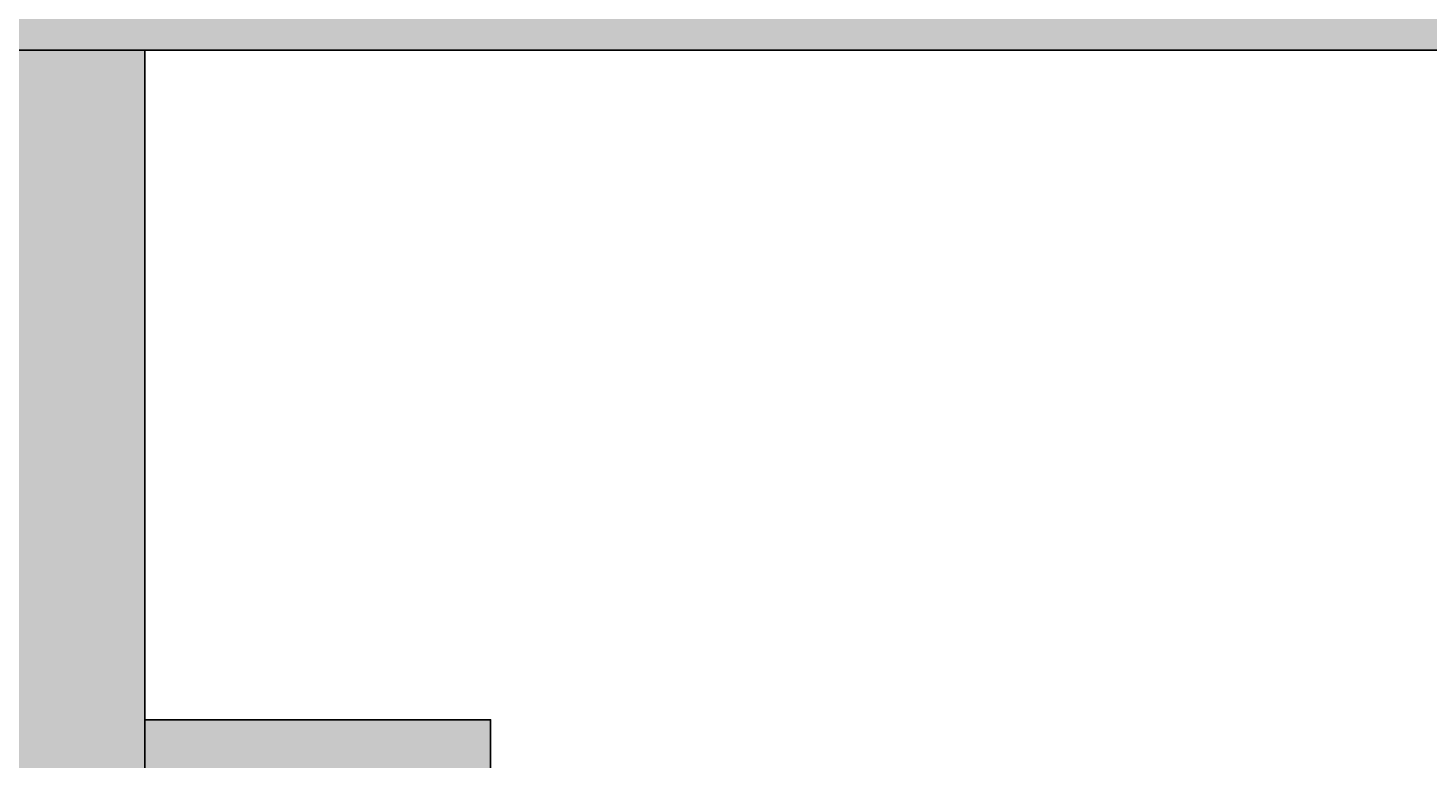
# Model space of a CAD drawing. Units: millimetres. Extents: x -11 to 280, y -4 to 208.
# Tile 34 of 55: x 189 to 222, y 88 to 106. Entities that reach past the tile are written whole.
import ezdxf

# ---------------------------------------------------------------- set-up
doc = ezdxf.new("R2010")
doc.units = ezdxf.units.MM
for name, color, linetype, lineweight in [('M-DIMS', 2, 'Continuous', 18), ('M-HYDR-PRES', 7, 'Continuous', 25), ('M-HYDR-VALV', 7, 'Continuous', 25), ('M-HYDR-VALV-PATT', 252, 'Continuous', 13)]:
    doc.layers.add(name, color=color, linetype=linetype, lineweight=lineweight)
doc.layers.add('M-HYDR-PRES-PATT', color=240, linetype='Continuous', lineweight=13, true_color=0xed1f24)
doc.styles.get("Standard").update_dxf_attribs({"font": 'arial.ttf'})
doc.dimstyles.get("Standard").update_dxf_attribs({"dimtxt": 0.18, "dimasz": 0.18, "dimexe": 0.18, "dimexo": 0.0625, "dimgap": 0.09, "dimtad": 0, "dimtih": 1, "dimtoh": 1, "dimdec": 4, "dimzin": 0, "dimdsep": 46, "dimtxsty": 'Standard', "dimcen": 0.09, "dimadec": 0, "dimazin": 0, "dimtfac": 1, "dimtdec": 4, "dimtofl": 0, "dimtmove": 0, "dimatfit": 3, "dimfxl": 1, "dimtolj": 1, "dimtzin": 0, "dimarcsym": 0})

# ---------------------------------------------------------------- blocks, each defined once
blk = doc.blocks.new('*D5')
at = {"layer": 'Defpoints', "color": 0, "transparency": 16777216}
for p in [(24.759, 192.645), (-10.087, 11.435), (261.686, 11.435)]:
    blk.add_point(p, dxfattribs=at)
at = {"layer": 'M-DIMS', "color": 0, "lineweight": -2, "transparency": 16777216}
for p, q in [((24.696, 192.645), (-10.267, 192.645)), ((-10.087, 192.465), (-10.087, 102.222)), ((-10.087, 11.615), (-10.087, 101.858)), ((261.624, 11.435), (-10.267, 11.435))]:
    blk.add_line(p, q, dxfattribs=at)
at = {"layer": 'M-DIMS', "color": 0, "transparency": 16777216}
for points in [[(-10.117, 192.465), (-10.057, 192.465), (-10.087, 192.645)], [(-10.117, 11.615), (-10.057, 11.615), (-10.087, 11.435)]]:
    blk.add_solid(points, dxfattribs=at)
at = {"layer": 'M-DIMS', "color": 0, "transparency": 16777216, "insert": (-10.087, 102.04), "char_height": 0.18, "attachment_point": 5}
blk.add_mtext('\\A1;181.2', dxfattribs=at)
blk = doc.blocks.new('*D13')
at = {"layer": 'Defpoints', "color": 0, "transparency": 16777216}
for p in [(191.774, 105.314), (232.2, 105.314), (232.2, -3.415)]:
    blk.add_point(p, dxfattribs=at)
at = {"layer": 'M-DIMS', "color": 0, "lineweight": -2, "transparency": 16777216}
for p, q in [((191.774, 105.252), (191.774, -3.595)), ((232.2, 105.252), (232.2, -3.595)), ((191.954, -3.415), (211.52, -3.415)), ((232.02, -3.415), (212.454, -3.415))]:
    blk.add_line(p, q, dxfattribs=at)
at = {"layer": 'M-DIMS', "color": 0, "transparency": 16777216}
for points in [[(191.954, -3.385), (191.954, -3.445), (191.774, -3.415)], [(232.02, -3.385), (232.02, -3.445), (232.2, -3.415)]]:
    blk.add_solid(points, dxfattribs=at)
at = {"layer": 'M-DIMS', "color": 0, "transparency": 16777216, "insert": (211.987, -3.415), "char_height": 0.18, "attachment_point": 5}
blk.add_mtext('\\A1;40.426', dxfattribs=at)
blk = doc.blocks.new('*D20')
at = {"layer": 'Defpoints', "color": 0, "transparency": 16777216}
for p in [(231.68, 207.495), (151.022, 43.599), (231.68, 43.599)]:
    blk.add_point(p, dxfattribs=at)
at = {"layer": 'M-DIMS', "color": 0, "lineweight": -2, "transparency": 16777216}
for p, q in [((151.022, 43.662), (151.022, 207.675)), ((231.68, 43.662), (231.68, 207.675)), ((151.202, 207.495), (190.957, 207.495)), ((231.5, 207.495), (191.745, 207.495))]:
    blk.add_line(p, q, dxfattribs=at)
at = {"layer": 'M-DIMS', "color": 0, "transparency": 16777216}
for points in [[(151.202, 207.525), (151.202, 207.465), (151.022, 207.495)], [(231.5, 207.525), (231.5, 207.465), (231.68, 207.495)]]:
    blk.add_solid(points, dxfattribs=at)
at = {"layer": 'M-DIMS', "color": 0, "transparency": 16777216, "insert": (191.351, 207.495), "char_height": 0.18, "attachment_point": 5}
blk.add_mtext('\\A1;80.66', dxfattribs=at)

msp = doc.modelspace()

# ---------------------------------------------------------------- hatches: boundary and pattern name
at = {"layer": 'M-HYDR-PRES-PATT'}
h = msp.add_hatch(color=256, dxfattribs=at)
h.set_gradient(color1=(237, 31, 36), color2=(237, 31, 36), tint=1)
h.paths.add_polyline_path([(232.2, 133.1228), (228.7, 133.1228), (228.7, 108.8141), (102.7646, 108.8141), (102.7646, 105.3141), (232.2, 105.3141)])
h.paths.add_polyline_path([(128.8433, 105.3141), (125.3433, 105.3141), (125.3433, 91.7099, 1), (128.8433, 91.7099)])
h.paths.add_polyline_path([(229.1617, 78.7098), (196.7745, 78.7098, -0.4142136), (191.7745, 83.7098), (191.7745, 105.3141), (188.2745, 105.3141), (188.2745, 80.2098, 0.4142136), (193.2745, 75.2098), (225.6617, 75.2098), (225.6617, 43.5991), (229.1617, 43.5991)])
h.paths.add_polyline_path([(102.7646, 110.3704), (95.5776, 110.3704), (95.5776, 103.9022), (102.7646, 103.9022)])
h.paths.add_polyline_path([(100.7059, 107.2502), (99.1711, 106.3641), (99.1711, 106.8641), (97.1711, 106.8641), (97.1711, 107.6363), (99.1711, 107.6363), (99.1711, 108.1363)], flags=16)
h.paths.add_polyline_path([(234.6119, 138.4081), (226.5106, 138.4081), (226.5106, 133.1228), (234.6119, 133.1228)])
h.paths.add_polyline_path([(231.1963, 135.7055), (230.2965, 134.1786), (229.4241, 135.7213), (229.9241, 135.7168), (229.9418, 137.7167), (230.7141, 137.7099), (230.6963, 135.71)], flags=16)
at = {"layer": 'M-HYDR-VALV-PATT'}
h = msp.add_hatch(color=256, dxfattribs=at)
h.set_gradient(color1=(153, 27, 30), color2=(153, 27, 30), tint=1)
h.paths.add_polyline_path([(131.8437, 88.2421, -0.3394543), (132.5849, 89.208), (121.2548, 86.1721, -0.4931454), (122.5137, 85.2062, -0.3394543), (121.7725, 84.2403), (133.1025, 87.2762, -0.4931454)])
h.paths.add_polyline_path([(133.1025, 83.1351, -0.4931454), (131.8437, 84.101, -0.3394543), (132.5849, 85.0669), (121.2548, 82.031, -0.4931454), (122.5137, 81.0651, -0.3394543), (121.7725, 80.0992)])
h.paths.add_polyline_path([(133.1025, 78.994, -0.4931454), (131.8437, 79.9599, -0.3394543), (132.5849, 80.9258), (121.2548, 77.8899, -0.4931454), (122.5137, 76.924, -0.3394543), (121.7725, 75.9581)])
h.paths.add_polyline_path([(197.7905, 78.7098), (200.0003, 78.7098), (200.0003, 89.3873), (191.7745, 89.3873), (191.7745, 87.1776, -0.2439164)])
h.paths.add_polyline_path([(200.0003, 65.0638), (200.0003, 75.2098), (197.7325, 75.2098, -0.4135811), (184.7092, 66.0277), (184.7092, 65.0638)])
h.paths.add_polyline_path([(181.2092, 65.0638), (181.2092, 67.2471, -0.2598454), (175.3563, 76.54), (173.8038, 76.54), (173.8038, 65.0638)])
h.paths.add_polyline_path([(188.2745, 88.3022), (188.2745, 89.3873), (173.8038, 89.3873), (173.8038, 80.04), (175.7181, 80.04, -0.3816661)])

# ---------------------------------------------------------------- linework, layer by layer
at = {"layer": 'M-HYDR-PRES'}
msp.add_lwpolyline([(232.2, 133.1228), (232.2, 105.3141), (102.7646, 105.3141)], dxfattribs=at)
msp.add_lwpolyline([(191.7745, 105.3141), (191.7745, 83.7098, 0.4142136), (196.7745, 78.7098), (229.1617, 78.7098), (229.1617, 43.5991)], format="xyb", dxfattribs=at)
at = {"layer": 'M-HYDR-VALV'}
msp.add_lwpolyline([(191.7745, 89.3873), (200.0003, 89.3873), (200.0003, 78.7098)], dxfattribs=at)

# ---------------------------------------------------------------- dimensions: what is measured, and where the dimension line sits
at = {"layer": 'M-DIMS'}
for base, p1, p2, override, picture, middle in [((231.6803, 207.495), (151.0217, 43.5991), (231.6803, 43.5991), {"dimdec": 2, "dimlfac": 1, "dimrnd": 0, "dimzin": 0, "dimdsep": 46, "dimlunit": 2}, '*D20', (191.351, 207.495)), ((232.20002, -3.41542), (191.77448, 105.31407), (232.20002, 105.31407), {"dimdec": 3, "dimlfac": 1, "dimrnd": 0, "dimzin": 0, "dimdsep": 46, "dimlunit": 2}, '*D13', (211.98725, -3.41542))]:
    dim = msp.add_linear_dim(base=base, p1=p1, p2=p2, dimstyle='Standard', override=override, dxfattribs=at)
    dim.commit()
    dim.dimension.update_dxf_attribs({"geometry": picture, "text_midpoint": middle})
dim = msp.add_linear_dim(base=(-10.0865, 11.4346), p1=(24.7588, 192.645), p2=(261.6863, 11.4346), angle=90, dimstyle='Standard', override={"dimdec": 1, "dimlfac": 1, "dimrnd": 0, "dimzin": 0, "dimdsep": 46, "dimlunit": 2}, dxfattribs=at)
dim.commit()
dim.dimension.update_dxf_attribs({"geometry": '*D5', "text_midpoint": (-10.0865, 102.0398)})

doc.saveas('drawing.dxf')
